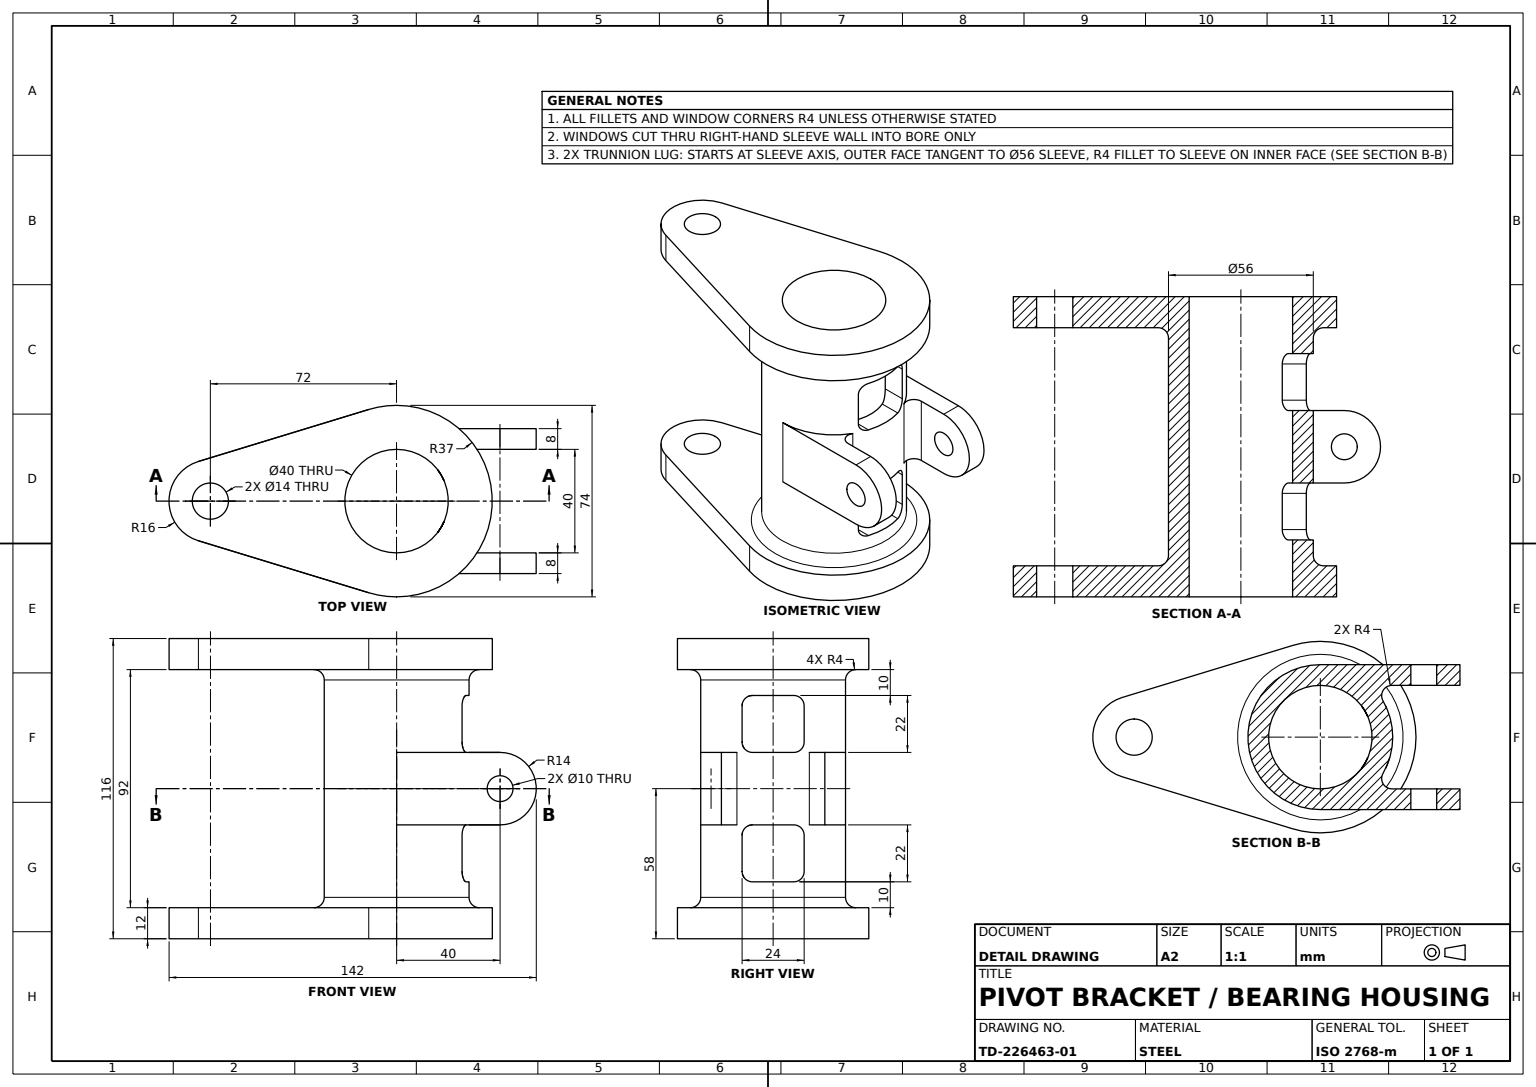
SolidWorks part; units mm, degrees
material "Plain Carbon Steel"
ref_plane "Front Plane" through (0, 0, 0) normal (0, 0, 1) x (1, 0, 0)
ref_plane "Top Plane" through (0, 0, 0) normal (0, 1, 0) x (1, 0, 0)
ref_plane "Right Plane" through (0, 0, 0) normal (1, 0, 0) x (0, 0, -1)
sketch "Lower Arm Profile" plane through (0, 0, 0) normal (0, 1, 0) x (1, 0, 0)
  line L0 (-76.6667, 15.3043) -> (-10.7917, 35.3912)
  line L1 (-76.6667, -15.3043) -> (-10.7917, -35.3912)
  arc A0 (-10.7917, -35.3912) -> (-10.7917, 35.3912) centre (0, 0) ccw
  arc A1 (-76.6667, 15.3043) -> (-76.6667, -15.3043) centre (-72, 0) ccw
  circle A2 centre (-72, 0) radius 7
  dimension "D1" = 16
  dimension "D2" = 37
  dimension "D4" = 14
  dimension "D3" = 72
extrude "Lower Arm Plate" add sketch "Lower Arm Profile" along normal blind 12
sketch "Sleeve Profile Ø56" plane through (0, 12, 0) normal (0, 1, 0) x (1, 0, 0)
  circle A0 centre (0, 0) radius 28
  dimension "D1" = 56
extrude "Sleeve Ø56" add sketch "Sleeve Profile Ø56" along normal blind 92
ref_plane "Arm Mirror Plane" through (0, 58, 0) normal (0, 1, 0) x (1, 0, 0)
mirror "Upper Arm Mirror" about plane through (0, 58, 0) normal (0, 1, 0) of "Lower Arm Plate"
fillet "Arm Fillets R4" radius 4 2 edges at (0, 12, 28) (0, 104, 28)
sketch "Trunnion Lug Profile" plane through (0, 0, 0) normal (0, 0, 1) x (1, 0, 0)
  line L0 (0, 72) -> (40, 72)
  line L1 (40, 44) -> (0, 44)
  line L2 (0, 44) -> (0, 72)
  arc A0 (40, 72) -> (40, 44) centre (40, 58) cw
  circle A1 centre (40, 58) radius 5
  dimension "D3" = 14
  dimension "D4" = 10
  dimension "D1" = 40
  dimension "D2" = 58
extrude "Trunnion Lug" add sketch "Trunnion Lug Profile" along normal blind 8 from offset 20
mirror "Trunnion Lug Mirror" about plane through (0, 0, 0) normal (0, 0, 1) of "Trunnion Lug"
fillet "Lug Fillets R4" radius 4 2 edges at (19.5959, 58, -20) (19.5959, 58, 20)
sketch "Sleeve Window Profile" plane through (0, 0, 0) normal (1, 0, 0) x (0, 0, -1)
  line L0 (28, 72) -> (14, 72) construction
  line L1 (-8, 94) -> (8, 94)
  line L2 (-12, 90) -> (-12, 76)
  line L3 (-8, 72) -> (8, 72)
  line L4 (12, 90) -> (12, 76)
  line L5 (-28, 58) -> (25.0441, 58) construction
  line L6 (-28, 72) -> (-28, 44) construction
  line L7 (-8, 22) -> (8, 22)
  line L8 (12, 26) -> (12, 40)
  line L9 (-8, 44) -> (8, 44)
  line L10 (-12, 26) -> (-12, 40)
  line L11 (14, 44) -> (28, 44) construction
  arc A0 (-12, 76) -> (-8, 72) centre (-8, 76) ccw
  arc A1 (8, 72) -> (12, 76) centre (8, 76) ccw
  arc A2 (8, 94) -> (12, 90) centre (8, 90) cw
  arc A3 (-8, 94) -> (-12, 90) centre (-8, 90) ccw
  arc A4 (8, 22) -> (12, 26) centre (8, 26) ccw
  arc A5 (-12, 40) -> (-8, 44) centre (-8, 40) cw
  arc A6 (8, 44) -> (12, 40) centre (8, 40) cw
  arc A7 (-8, 22) -> (-12, 26) centre (-8, 26) cw
  point P7 (0, 72)
  dimension "D3" = 4
  dimension "D1" = 22
  dimension "D2" = 24
extrude "Sleeve Windows" cut sketch "Sleeve Window Profile" along normal through all
sketch "Bore Profile Ø40" plane through (0, 116, 0) normal (0, 1, 0) x (1, 0, 0)
  circle A0 centre (0, 0) radius 20
  dimension "D1" = 40
extrude "Bore Ø40" cut sketch "Bore Profile Ø40" against normal through all
